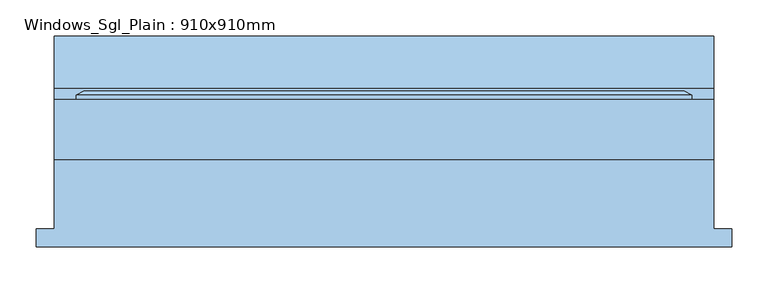
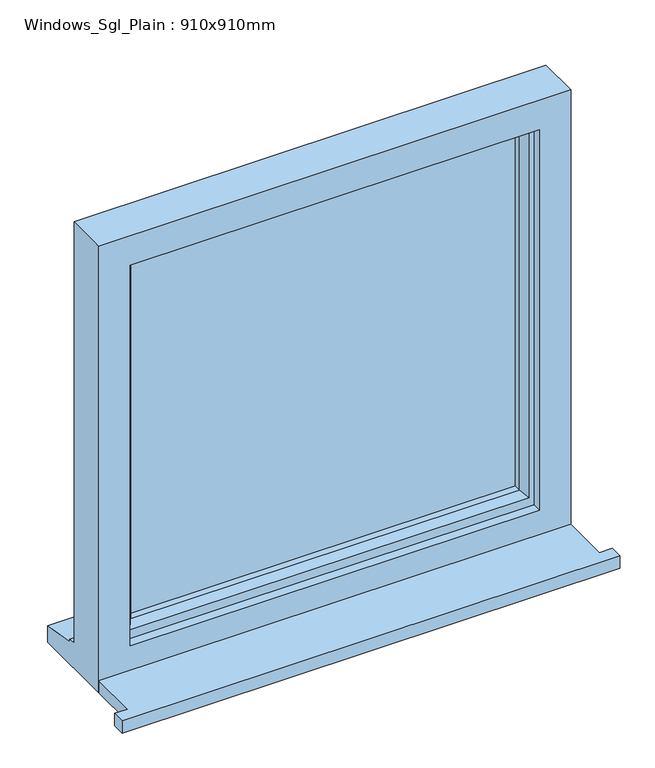
"""IFC4 building model written with IfcOpenShell, lengths in millimetres: window geometry, Windows_Sgl_Plain : 910x910mm."""

from ifc_helpers import new_model, si_unit, frame, origin, place, context, project, spatial, polyline, outline, extrude, faceted_brep, source, transform, mapped, element, save


def windows_sgl_plain_910x910mm_ba4b8fff(model_context):
    return source(origin(), model_context, "Body", "SolidModel", [
        extrude(outline(polyline([(-480.0, -130.8434322), (-480.0, -105.8434322), (-455.0, -105.8434322), (-455.0, -10.2434322), (455.0, -10.2434322), (455.0, -105.8434322), (480.0, -105.8434322), (480.0, -130.8434322), (-480.0, -130.8434322)])), frame((0.0, 0.0, 1200.0), z_axis=(0.0, 0.0, 1.0), x_axis=(1.0, 0.0, 0.0)), (0.0, 0.0, 1.0), 25.0),
        faceted_brep([(-455.0, -10.2434322, 1200.0), (455.0, -10.2434322, 1200.0), (455.0, -10.2434322, 2110.0), (-455.0, -10.2434322, 2110.0), (-395.0, -10.2434322, 2050.0), (395.0, -10.2434322, 2050.0), (395.0, -10.2434322, 1275.0), (-395.0, -10.2434322, 1275.0), (-455.0, 72.7565678, 2110.0), (-455.0, 72.7565678, 1251.0), (-455.0, 87.7565678, 1249.68767), (-455.0, 87.7565678, 1244.7449676), (-455.0, 160.2565678, 1233.8088847), (-455.0, 160.2565678, 1200.0), (455.0, 72.7565678, 2110.0), (455.0, 72.7565678, 1251.0), (-415.0, 72.7565678, 2070.0), (-415.0, 72.7565678, 1263.0), (415.0, 72.7565678, 1263.0), (415.0, 72.7565678, 2070.0), (-415.0, 7.7565678, 2070.0), (-415.0, 7.7565678, 1263.0), (415.0, 7.7565678, 2070.0), (415.0, 7.7565678, 1263.0), (-395.0, 7.7565678, 2050.0), (-395.0, 7.7565678, 1275.0), (395.0, 7.7565678, 1275.0), (395.0, 7.7565678, 2050.0), (455.0, 160.2565678, 1200.0), (455.0, 160.2565678, 1233.8088847), (455.0, 87.7565678, 1244.7449676), (455.0, 87.7565678, 1249.68767)], [[[0, 1, 2, 3], [4, 5, 6, 7]], [[0, 3, 8, 9, 10, 11, 12, 13]], [[9, 8, 14, 15], [16, 17, 18, 19]], [[17, 16, 20, 21]], [[20, 22, 23, 21], [24, 25, 26, 27]], [[24, 4, 7, 25]], [[3, 2, 14, 8]], [[16, 19, 22, 20]], [[5, 4, 24, 27]], [[15, 14, 2, 1, 28, 29, 30, 31]], [[19, 18, 23, 22]], [[5, 27, 26, 6]], [[28, 1, 0, 13]], [[29, 28, 13, 12]], [[30, 29, 12, 11]], [[31, 30, 11, 10]], [[15, 31, 10, 9]], [[21, 23, 18, 17]], [[7, 6, 26, 25]]]),
        extrude(outline(polyline([(385.0, 36.7565678), (-385.0, 36.7565678), (-385.0, 60.7565678), (385.0, 60.7565678), (385.0, 36.7565678)])), frame((0.0, 0.0, 1293.0), z_axis=(0.0, 0.0, 1.0), x_axis=(1.0, 0.0, 0.0)), (0.0, 0.0, 1.0), 747.0),
        faceted_brep([(-425.0, 72.7565678, 2080.0), (-425.0, 78.5300705, 2080.0), (-425.0, 78.5300705, 1253.0), (-425.0, 72.7565678, 1253.0), (-415.0, 7.7565678, 2070.0), (-415.0, 72.7565678, 2070.0), (-415.0, 72.7565678, 1263.0), (-415.0, 7.7565678, 1263.0), (-375.0, 22.2494677, 2030.0), (-385.1480377, 7.7565678, 2040.1480377), (-385.1480377, 7.7565678, 1292.8519623), (-375.0, 22.2494677, 1303.0), (-375.0, 36.7565678, 2030.0), (-375.0, 36.7565678, 1303.0), (-385.0, 60.7565678, 2040.0), (-385.0, 36.7565678, 2040.0), (-385.0, 36.7565678, 1293.0), (-385.0, 60.7565678, 1293.0), (-375.0, 78.5300705, 2030.0), (-375.0, 60.7565678, 2030.0), (-375.0, 60.7565678, 1303.0), (-375.0, 78.5300705, 1303.0), (-392.4457548, 84.3035732, 2047.4457548), (-392.4457548, 84.3035732, 1285.5542452), (-414.2153903, 84.3035732, 2069.2153903), (-414.2153903, 84.3035732, 1263.7846097), (425.0, 78.5300705, 1253.0), (425.0, 72.7565678, 1253.0), (415.0, 72.7565678, 1263.0), (415.0, 7.7565678, 1263.0), (385.1480377, 7.7565678, 1292.8519623), (375.0, 22.2494677, 1303.0), (375.0, 36.7565678, 1303.0), (385.0, 36.7565678, 1293.0), (385.0, 60.7565678, 1293.0), (375.0, 60.7565678, 1303.0), (375.0, 78.5300705, 1303.0), (392.4457548, 84.3035732, 1285.5542452), (414.2153903, 84.3035732, 1263.7846097), (425.0, 78.5300705, 2080.0), (425.0, 72.7565678, 2080.0), (415.0, 72.7565678, 2070.0), (415.0, 7.7565678, 2070.0), (385.1480377, 7.7565678, 2040.1480377), (375.0, 22.2494677, 2030.0), (375.0, 36.7565678, 2030.0), (385.0, 36.7565678, 2040.0), (385.0, 60.7565678, 2040.0), (375.0, 60.7565678, 2030.0), (375.0, 78.5300705, 2030.0), (392.4457548, 84.3035732, 2047.4457548), (414.2153903, 84.3035732, 2069.2153903)], [[[0, 1, 2, 3]], [[4, 5, 6, 7]], [[8, 9, 10, 11]], [[12, 8, 11, 13]], [[14, 15, 16, 17]], [[18, 19, 20, 21]], [[22, 18, 21, 23]], [[1, 24, 25, 2]], [[3, 2, 26, 27]], [[7, 6, 28, 29]], [[11, 10, 30, 31]], [[13, 11, 31, 32]], [[17, 16, 33, 34]], [[21, 20, 35, 36]], [[23, 21, 36, 37]], [[2, 25, 38, 26]], [[27, 26, 39, 40]], [[29, 28, 41, 42]], [[31, 30, 43, 44]], [[32, 31, 44, 45]], [[34, 33, 46, 47]], [[36, 35, 48, 49]], [[37, 36, 49, 50]], [[26, 38, 51, 39]], [[40, 39, 1, 0]], [[3, 27, 40, 0], [5, 41, 28, 6]], [[42, 41, 5, 4]], [[7, 29, 42, 4], [9, 43, 30, 10]], [[44, 43, 9, 8]], [[45, 44, 8, 12]], [[15, 46, 33, 16], [13, 32, 45, 12]], [[47, 46, 15, 14]], [[17, 34, 47, 14], [19, 48, 35, 20]], [[49, 48, 19, 18]], [[50, 49, 18, 22]], [[24, 51, 38, 25], [23, 37, 50, 22]], [[39, 51, 24, 1]]]),
    ])


if __name__ == "__main__":
    model = new_model("IFC4")
    model_context = context("Model", 3, world=origin())
    ifc_project = project(units=[si_unit("LENGTHUNIT", "METRE", prefix="MILLI")], contexts=[model_context])
    site = spatial("IfcSite", under=ifc_project)
    building = spatial("IfcBuilding", under=site)
    placement = place(None, origin())
    windows_sgl_plain_910x910mm_shape = windows_sgl_plain_910x910mm_ba4b8fff(model_context)
    element("IfcWindow", 1, ObjectType="Windows_Sgl_Plain : 910x910mm", at=placement, inside=building, context=model_context, shape_type="MappedRepresentation", body=[
        mapped(windows_sgl_plain_910x910mm_shape, transform((0.0, 0.0, 0.0), x_axis=(1.0, 0.0, 0.0), y_axis=(0.0, 1.0, 0.0), z_axis=(0.0, 0.0, 1.0))),
    ])
    save(model, "model.ifc")

# Revit data of these elements
# Type "Windows_Sgl_Plain : 910x910mm"
#   Type Mark = "44"
#   Operation = "SinglePanel"
#   Construction Type Id = "SGL"
#   Manufacturer = "Revit"
#   Keynote = "L10"
#   Analytic Construction = "Large single-glazed windows"
#   Wrap Layers (Ext) from Ext = 102.5 mm
#   Wrap Layers (Int) from Ext = 177.5 mm
#   Window Board Projection = 25 mm
#   Window Board Extension = 25 mm
#   Visual Light Transmittance = 0.9
#   Solar Heat Gain Coefficient = 0.86
#   Rough Width = 910 mm
#   Rough Height = 910 mm
#   Height = 910 mm
#   Width = 910 mm
#   Heat Transfer Coefficient (U) = 5.5617 W/(m²·K)
#   Glazing Thickness = 24 mm
#   FrameOffset - External = 50 mm
#   Frame Depth = 65 mm
#   Default Head Height = 2110 mm
#   Cill Depth = 87.5 mm
#   Cavity Closer Width = 50 mm
#   Cavity Closer Offset from Ext = 102.5 mm
#   Cavity Closer Depth = 85 mm
#   Define Thermal Properties by = 1
#   Vis - Cavity Closers = yes
#   Define Thermal Properties by = 1
#   Material Trim = Window Frame
#   Material Glass = Glass
#   Material Frame = Window Frame
#   Wall Closure = (empty or 0)
# Element 1 (IfcWindow, "Windows_Sgl_Plain : 910x910mm")
#   Materials on its faces: "Window Frame", "Glass"
# Materials
#   "Window Frame": colour RGB 249 249 249, transparency 0, Keynote = "L10", Cost = 0
#   "Glass": class "Glass", colour RGB 0 128 192, transparency 0.9, Description = "Soda Lime Glass", Cost = 0
